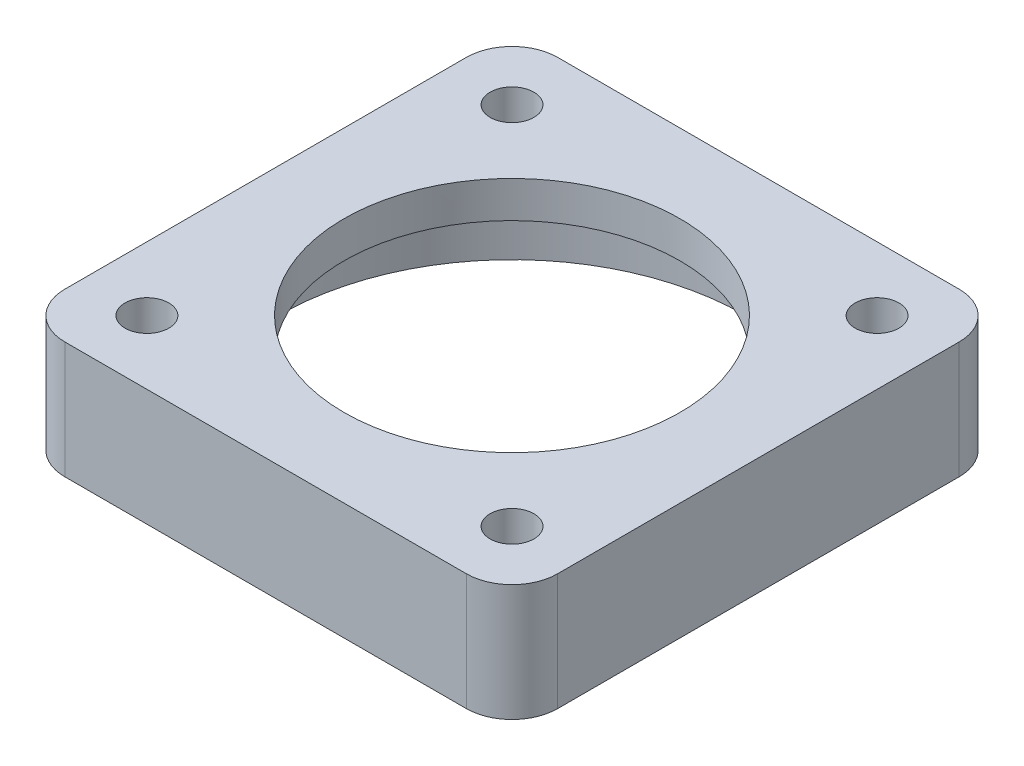
from build123d import *

# Parameters (mm, degrees)
BASE_PLATE_PROFILE_R        = 6
BASE_PLATE_135X135X32_DEPTH = 32
THROUGH_BORE_92_REACH       = 102.68
THROUGH_BORE_PROFILE_R      = 46
COUNTERBORE_PROFILE_R       = 64
COUNTERBORE_128X22_DEPTH    = 22


with BuildPart() as part:
    # Base Plate Profile → Base Plate 135x135x32 (new body)
    with BuildSketch(Plane(origin=(0, 0, 0), x_dir=(1, 0, 0), z_dir=(0, 1, 0))):
        with BuildLine():
            Line((-55, 67.5), (55, 67.5))
            ThreePointArc((55, 67.5), (63.838834765, 63.838834765), (67.5, 55))
            Line((67.5, 55), (67.5, -55))
            ThreePointArc((67.5, -55), (63.838834765, -63.838834765), (55, -67.5))
            Line((55, -67.5), (-55, -67.5))
            ThreePointArc((-55, -67.5), (-63.838834765, -63.838834765), (-67.5, -55))
            Line((-67.5, -55), (-67.5, 55))
            ThreePointArc((-67.5, 55), (-63.838834765, 63.838834765), (-55, 67.5))
        make_face()
        with Locations(Location((-50, 50, 0), (0, 0, 270))):
            Circle(BASE_PLATE_PROFILE_R, mode=Mode.SUBTRACT)
        with Locations(Location((50, 50, 0), (0, 0, 90))):
            Circle(BASE_PLATE_PROFILE_R, mode=Mode.SUBTRACT)
        with Locations(Location((50, -50, 0), (0, 0, 270))):
            Circle(BASE_PLATE_PROFILE_R, mode=Mode.SUBTRACT)
        with Locations(Location((-50, -50, 0), (0, 0, 90))):
            Circle(BASE_PLATE_PROFILE_R, mode=Mode.SUBTRACT)
    extrude(amount=BASE_PLATE_135X135X32_DEPTH)

    # Through Bore Profile → Through Bore Ø92 (cut, up to next)
    with BuildSketch(Plane(origin=(0, 32, 0), x_dir=(1, 0, 0), z_dir=(0, 1, 0)), mode=Mode.PRIVATE) as through_bore_92_sk1:
        with Locations(Location((0, 0, 0), (0, 0, 270))):
            Circle(THROUGH_BORE_PROFILE_R)
    through_bore_92_tool1 = extrude(through_bore_92_sk1.sketch, amount=-THROUGH_BORE_92_REACH, mode=Mode.PRIVATE) & part.part
    add(through_bore_92_tool1.solids().sort_by_distance((0, 32, 0))[0], mode=Mode.SUBTRACT)

    # Counterbore Profile → Counterbore Ø128x22 (cut)
    with BuildSketch(Plane(origin=(0, 0, 0), x_dir=(-1, 0, 0), z_dir=(0, -1, 0))):
        with Locations(Location((0, 0, 0), (0, 0, 90))):
            Circle(COUNTERBORE_PROFILE_R)
    extrude(amount=-COUNTERBORE_128X22_DEPTH, mode=Mode.SUBTRACT)


solid = part.part
